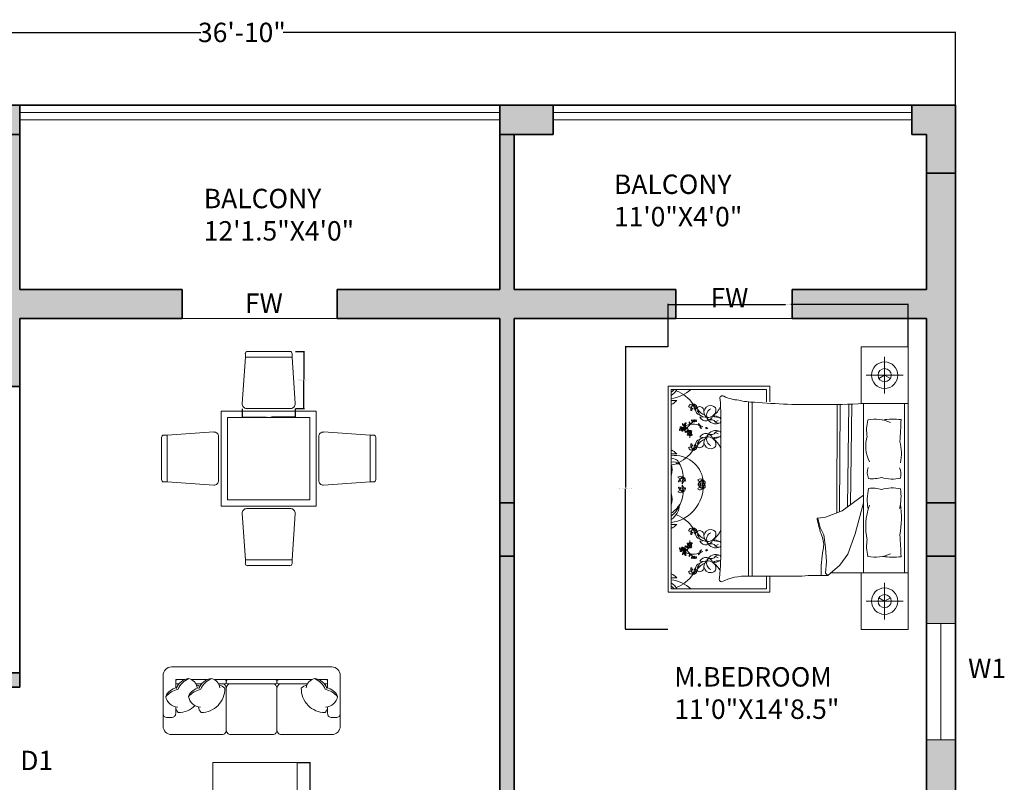
# Model space of a CAD drawing. Units: inches. Extents: x -9 to 505, y -680 to 48.
# Tile 17 of 17: x 179 to 484, y -198 to 38. Entities that reach past the tile are written whole.
import ezdxf

# ---------------------------------------------------------------- set-up
doc = ezdxf.new("R2010")
doc.units = ezdxf.units.IN
doc.header["$MEASUREMENT"] = 0
for name, color, linetype, lineweight in [('A-ANNO-DIMS', 2, 'Continuous', 18), ('A-ANNO-TEXT', 7, 'Continuous', 18), ('A-AREA-IDEN', 7, 'Continuous', 18), ('A-FLOR-HRAL', 4, 'Continuous', 18), ('A-FURN', 8, 'Continuous', 18), ('A-GLAZ', 4, 'Continuous', 18), ('A-WALL', 7, 'Continuous', 35), ('A-WALL-PATT', 251, 'Continuous', 13), ('S-CONC', 7, 'Continuous', 35), ('S-CONC-PATT', 18, 'Continuous', 13)]:
    doc.layers.add(name, color=color, linetype=linetype, lineweight=lineweight)
doc.styles.get("Standard").update_dxf_attribs({"font": 'arial.ttf'})
doc.dimstyles.get("Standard").update_dxf_attribs({"dimtxt": 0.18, "dimasz": 0.18, "dimexe": 0.18, "dimexo": 0.0625, "dimgap": 0.09, "dimtad": 0, "dimtih": 1, "dimtoh": 1, "dimdec": 0, "dimzin": 0, "dimdsep": 46, "dimlunit": 3, "dimtxsty": 'Standard', "dimcen": 0.09, "dimadec": 0, "dimazin": 0, "dimtfac": 1, "dimtdec": 0, "dimtofl": 0, "dimtmove": 0, "dimatfit": 3, "dimfxl": 1, "dimtolj": 1, "dimtzin": 0, "dimarcsym": 0})

# ---------------------------------------------------------------- blocks, each defined once
blk = doc.blocks.new('*D2')
at = {"layer": 'A-ANNO-DIMS', "color": 0, "lineweight": -2, "transparency": 16777216}
for p, q in [((27.26, 11.56), (27.26, 34.2)), ((27.44, 34.02), (235.29, 34.02)), ((468.58, 34.02), (260.74, 34.02)), ((468.76, 11.56), (468.76, 34.2))]:
    blk.add_line(p, q, dxfattribs=at)
at = {"layer": 'A-ANNO-DIMS', "color": 0, "transparency": 16777216}
for points in [[(27.44, 34.05), (27.44, 33.99), (27.26, 34.02)], [(468.58, 34.05), (468.58, 33.99), (468.76, 34.02)]]:
    blk.add_solid(points, dxfattribs=at)
at = {"layer": 'Defpoints', "color": 0, "transparency": 16777216}
for p in [(468.76, 34.02), (27.26, 11.5), (468.76, 11.5)]:
    blk.add_point(p, dxfattribs=at)
at = {"layer": 'A-ANNO-DIMS', "color": 0, "transparency": 16777216, "insert": (248.01, 34.02), "char_height": 6, "attachment_point": 5}
blk.add_mtext('\\A1;36\'-10"', dxfattribs=at)
blk = doc.blocks.new('BED-DOUBLE-WITH-NIGHTSTANDS')
for p, q in [((74.3, 0), (74.3, 87.37)), ((67.02, 72.93), (67.02, 84.34)), ((61.31, 78.63), (72.73, 78.63)), ((0, 75.23), (0, 11.53)), ((31.47, 75.23), (0, 75.23)), ((1.01, 74.22), (30.46, 74.22)), ((1.01, 12.54), (1.01, 74.22)), ((30.46, 74.22), (30.46, 70.37)), ((31.47, 70.38), (31.47, 75.23)), ((24.93, 70.38), (24.93, 16.47)), ((26.02, 70.29), (26.02, 16.47)), ((52.32, 69.59), (52.18, 36.06)), ((53.22, 69.58), (53.09, 36.41)), ((55.97, 69.63), (55.52, 37.9)), ((56.87, 69.66), (56.43, 38.56)), ((60.5, 17.47), (60.5, 69.9)), ((73.18, 69.9), (73.18, 17.47)), ((9.87, 65.61), (10.86, 65.8)), ((16.35, 61.42), (16.35, 25.95)), ((9.87, 59.5), (10.86, 59.31)), ((60.5, 41.48), (53.83, 36.69)), ((53.83, 36.69), (48.7, 34.74)), ((57.9, 29.61), (60.5, 39.14)), ((48.7, 34.74), (46.4, 34.39)), ((46.4, 34.39), (47.11, 31.56)), ((47.11, 31.56), (48.17, 29.26)), ((9.87, 27.26), (10.86, 27.45)), ((48.17, 29.26), (48.7, 25.36)), ((55.6, 23.24), (57.9, 29.61)), ((48.7, 25.36), (49.06, 20.94)), ((53.12, 19.88), (55.6, 23.24)), ((9.87, 21.15), (10.86, 20.96)), ((49.06, 20.94), (48.7, 17.4)), ((49.41, 16.69), (53.12, 19.88)), ((30.46, 16.47), (30.46, 12.54)), ((31.47, 11.53), (31.47, 16.47)), ((48.7, 17.4), (49.41, 16.69)), ((74.3, 17.47), (50.32, 17.47)), ((30.46, 12.54), (1.01, 12.54)), ((67.02, 14.45), (67.02, 3.03)), ((0, 11.53), (31.47, 11.53)), ((61.31, 8.74), (72.73, 8.74))]:
    blk.add_line(p, q)
for points in [[(74.3, 69.9), (59.74, 69.9), (59.74, 87.37), (74.3, 87.37)], [(67.02, 78.63), (65.26, 77.62)], [(67.02, 78.63), (68.79, 77.62)], [(59.74, 17.47), (59.74, 0), (74.3, 0)], [(67.02, 8.74), (65.26, 9.76)], [(67.02, 8.74), (68.79, 9.76)]]:
    blk.add_lwpolyline(points)
for points in [[(26.71, 70.27, -0.056112), (21.91, 70.9, -0.095341), (17.28, 72.13)], [(72.13, 64.88, 0.074897), (66.42, 64.77, -0.472817)], [(66.1, 47.01, 0.14099), (71.92, 46.83, 0.235245)], [(66.1, 43.28, -0.14099), (71.92, 43.45, -0.235245)], [(72.13, 22.49, -0.074897), (66.42, 22.6, 0.472817)], [(41.41, 16.51, -0.001242), (24.83, 16.47, 0.127202), (16.57, 14.72)]]:
    blk.add_lwpolyline(points, format="xyb")
for centre, radius in [((67.02, 78.63), 4.08), ((67.02, 78.63), 2.04), ((4.36, 62.02), 0.223), ((6.7, 60.56), 0.223), ((4.36, 24.75), 0.223), ((6.7, 26.2), 0.223), ((67.02, 8.74), 4.08), ((67.02, 8.74), 2.04)]:
    blk.add_circle(centre, radius)
for centre, radius, start, end in [((-2.05, 76.99), 5.56, 303.4617, 330.1116), ((-3.09, 78.99), 6.93, 306.3036, 316.4814), ((-0.53, 82.71), 11.41, 277.745, 311.8856), ((-1.65, 63.19), 11.41, 34.3865, 68.5908), ((-0.77, 73.87), 4.64, 292.5547, 318.9546), ((1.73, 86.58), 15.79, 267.4081, 273.6519), ((16.83, 71.47), 0.796, 56.1736, 203.4781), ((-68.63, 64.1), 85.02, 358.1965, 4.7598), ((44.11, 274.32), 204.79, 265.1265, 270.8855), ((7.49, 68.4), 1.27, 77.7115, 159.0387), ((6.81, 69.66), 0.953, 238.4633, 358.2869), ((9.93, 67.74), 2.89, 138.8402, 177.9352), ((7.19, 67.84), 0.142, 177.9352, 11.4834), ((7.26, 67.85), 0.0688, 11.4834, 127.9409), ((8.2, 68.81), 0.933, 117.6827, 223.7762), ((7.66, 68.26), 0.0744, 223.7729, 159.7333), ((7.99, 68.72), 0.946, 2.9516, 103.728), ((15.55, 71.37), 7.98, 192.5173, 207.1824), ((6.71, 68.17), 1.8, 345.4653, 54.2343), ((9.43, 70.65), 1.95, 211.3827, 255.2969), ((9.8, 67.61), 1.31, 350.264, 160.8688), ((10.19, 67.92), 1.64, 175.969, 254.3045), ((8.38, 67.88), 0.804, 333.9755, 53.2681), ((8.02, 66.16), 1.74, 6.1662, 51.5825), ((12.69, 70.21), 4.12, 211.2614, 251.7045), ((13.16, 67.13), 2.09, 84.9449, 172.8857), ((13.63, 67.49), 2.54, 182.3591, 234.0401), ((13.96, 66.31), 2.03, 111.5819, 201.4221), ((12.28, 68.18), 2.63, 265.2933, 346.921), ((13.37, 67.73), 1.48, 354.4856, 91.0538), ((10.2, 71.58), 6.61, 303.6671, 336.3547), ((49.82, 226.53), 156.99, 269.0718, 273.9), ((8.96, 64.13), 2.46, 178.3264, 187.1302), ((6.3, 63.79), 0.459, 11.3256, 64.4621), ((7.86, 64.45), 1.38, 190.2588, 210.656), ((1.29, 69.52), 8.3, 313.1541, 322.0459), ((7.39, 64.54), 0.171, 142.4737, 265.053), ((7.61, 64.57), 0.367, 127.7621, 169.0403), ((7.42, 64.88), 0.517, 265.053, 338.3618), ((8.1, 64.17), 0.676, 113.4276, 137.6104), ((8.03, 64.87), 0.223, 183.2768, 356.7232), ((8.19, 64.47), 0.364, 139.7889, 227.6792), ((8.07, 64.34), 0.192, 227.6792, 350.3487), ((7.33, 64.48), 0.728, 353.0852, 15.7171), ((7.81, 64.39), 0.46, 350.3487, 43.6538), ((8.66, 64.86), 0.535, 198.7263, 262.5032), ((8.24, 64.61), 0.213, 1.1081, 91.8675), ((8.64, 64.5), 0.172, 255.2356, 54.9248), ((8.37, 64.57), 0.371, 11.5637, 52.6358), ((12.35, 70.24), 4.69, 236.2883, 266.5076), ((11.75, 66.69), 2.17, 209.9085, 343.1337), ((12.67, 65.32), 0.542, 167.3041, 285.1471), ((14.13, 62.72), 3.37, 122.7011, 126.3445), ((14.77, 66.35), 2.78, 199.2822, 299.1751), ((13.28, 63.06), 1.79, 41.5653, 105.1471), ((15.71, 69.16), 3.62, 238.8218, 280.751), ((14.13, 62.72), 3.37, 55.785, 94.7304), ((14.26, 66.77), 2.51, 277.436, 299.9149), ((15.59, 65.12), 1.31, 221.5653, 293.8354), ((15.39, 64.67), 1.05, 17.4186, 52.325), ((15.39, 64.67), 1.05, 314.4517, 343.3657), ((73.15, 61.76), 11.71, 165.1039, 191.0369), ((64.13, 53.75), 11.26, 65.1316, 101.7583), ((903.62, 16.72), 832.89, 176.68521, 177.14978), ((3.72, 61.68), 0.171, 142.4737, 265.053), ((3.95, 61.71), 0.367, 61.2196, 169.0403), ((3.75, 62.02), 0.517, 265.053, 338.3618), ((4.19, 62.47), 0.439, 157.4086, 261.4386), ((3.94, 62.48), 0.22, 58.0499, 135.6268), ((4.44, 61.32), 0.676, 113.4276, 137.6104), ((4.17, 62.34), 0.147, 172.906, 277.132), ((3.69, 62.07), 0.702, 14.7558, 58.0499), ((4.52, 61.61), 0.364, 139.7889, 227.6792), ((4.41, 61.49), 0.192, 227.6792, 350.3487), ((4.67, 62.26), 0.303, 36.1046, 181.4281), ((3.66, 61.62), 0.728, 353.0852, 15.7171), ((4.68, 63.45), 0.248, 124.3538, 214.3923), ((4.14, 61.53), 0.46, 350.3487, 43.6538), ((5.05, 63.41), 0.579, 190.3057, 287.1958), ((4.49, 62.5), 0.306, 270.0645, 331.1507), ((4.75, 62.43), 0.35, 221.8413, 265.7877), ((4.99, 62.01), 0.535, 198.7263, 262.5032), ((5.21, 63.62), 0.673, 176.9701, 248.2913), ((10.01, 67.17), 6.5, 212.6784, 216.3746), ((4.57, 61.76), 0.213, 1.1081, 91.8675), ((4.75, 62.29), 0.218, 263.7526, 41.7054), ((4.7, 61.71), 0.371, 11.5637, 86.365), ((4.99, 63.46), 0.257, 216.3746, 291.7548), ((7.26, 59.85), 3.63, 124.0033, 132.4917), ((4.97, 61.64), 0.172, 255.2356, 54.9248), ((3.53, 59.39), 3.88, 63.7819, 68.2913), ((5.6, 62.38), 0.616, 128.3208, 208.8162), ((5.6, 63.28), 0.579, 122.8155, 187.3992), ((5.71, 62.42), 0.737, 207.7043, 254.3516), ((5.16, 63.04), 0.194, 289.3605, 111.7548), ((5.3, 63.04), 0.194, 221.8703, 44.2646), ((6.18, 62.48), 1.01, 157.2305, 229.0635), ((5.86, 63.21), 0.673, 109.4799, 177.6828), ((5.84, 62.81), 0.597, 174.4544, 220.6188), ((5.23, 62), 1.01, 270.278, 342.111), ((5.91, 60.73), 0.717, 98.7227, 159.3375), ((5.55, 61.65), 0.737, 244.9899, 291.6373), ((2.45, 59.48), 4.35, 30.544, 49.818), ((5.5, 63.63), 0.248, 56.8636, 146.9021), ((5.62, 63.36), 0.257, 148.8844, 224.2646), ((4.84, 61.96), 0.717, 340.0041, 40.6188), ((10.97, 60.13), 6.5, 145.1882, 148.8844), ((7.26, 59.85), 3.63, 94.756, 119.2041), ((14.99, 54.63), 11.94, 132.2412, 142.1744), ((5.71, 62.03), 0.597, 278.7227, 324.8872), ((5.61, 61.55), 0.616, 290.5253, 358.5375), ((6.53, 61.01), 0.439, 157.4086, 261.4386), ((6.29, 61.03), 0.22, 58.0499, 135.6268), ((6.81, 61.72), 0.616, 182.8499, 266.1226), ((6.57, 62.16), 0.597, 231.7607, 277.9252), ((7.04, 62.26), 1.01, 214.5369, 286.3699), ((6.03, 60.62), 0.702, 14.7558, 58.0499), ((2.45, 59.48), 4.35, 23.0501, 23.8477), ((6.93, 63.89), 0.419, 188.3432, 274.2869), ((6.75, 60.86), 0.717, 37.3105, 97.9252), ((7.3, 64.12), 0.732, 210.656, 242.6341), ((7.01, 60.81), 0.303, 36.1046, 181.4281), ((7.85, 64.75), 1.4, 218.2101, 226.3071), ((6.83, 61.84), 0.737, 265.0106, 311.658), ((6.82, 63.57), 0.178, 325.7657, 67.4417), ((7.45, 56.25), 7.24, 73.5842, 93.8277), ((7.1, 60.84), 0.218, 263.7526, 41.7054), ((11.9, 63.61), 2.46, 178.3264, 187.1302), ((9.24, 63.27), 0.459, 11.3256, 64.4621), ((10.8, 63.93), 1.38, 190.2588, 210.656), ((9.87, 63.37), 0.419, 188.3432, 274.2869), ((10.24, 63.6), 0.732, 210.656, 242.6341), ((10.79, 64.23), 1.4, 218.2101, 226.3071), ((9.76, 63.05), 0.178, 325.7657, 67.4417), ((10.26, 62.72), 0.419, 147.5332, 233.4768), ((10.63, 62.94), 0.732, 179.1859, 211.164), ((9.92, 62.77), 0.178, 354.3784, 96.0543), ((7.45, 56.25), 7.24, 63.0032, 69.8941), ((11.19, 63.27), 1.38, 211.164, 231.5612), ((11.43, 64.4), 2.46, 234.6898, 243.4936), ((11.45, 63.13), 1.4, 195.5129, 203.6099), ((9.87, 62.21), 0.459, 357.3579, 50.4944), ((11.84, 62.3), 0.168, 12.7051, 190.4384), ((11.95, 62.32), 0.274, 190.4384, 10.4136), ((14.77, 58.76), 2.78, 60.8249, 160.7178), ((15.59, 59.99), 1.31, 66.1646, 138.4347), ((15.39, 60.44), 1.05, 23.2856, 45.5483), ((6.07, 60.22), 0.171, 142.4737, 265.053), ((6.29, 60.26), 0.367, 61.2196, 169.0403), ((6.1, 60.57), 0.517, 265.053, 338.3618), ((6.78, 59.86), 0.676, 113.4276, 137.6104), ((6.52, 60.89), 0.147, 172.906, 277.132), ((6.87, 60.16), 0.364, 139.7889, 227.6792), ((6.75, 60.03), 0.192, 227.6792, 350.3487), ((6.01, 60.16), 0.728, 353.0852, 15.7171), ((2.45, 59.48), 4.35, 357.1071, 4.7585), ((6.49, 60.07), 0.46, 350.3487, 43.6538), ((7.34, 60.55), 0.535, 198.7263, 262.5032), ((6.84, 61.04), 0.306, 270.0645, 331.1507), ((7.1, 60.97), 0.35, 221.8413, 265.7877), ((6.91, 60.3), 0.213, 1.1081, 91.8675), ((7.05, 60.25), 0.371, 11.5637, 86.365), ((7.31, 60.19), 0.172, 255.2356, 54.9248), ((10.19, 57.19), 1.64, 105.6955, 184.031), ((8.02, 58.95), 1.74, 308.4175, 353.8338), ((12.69, 54.9), 4.12, 108.2955, 148.7386), ((12.35, 54.86), 4.69, 93.4924, 123.7117), ((11.75, 58.42), 2.17, 16.8663, 150.0915), ((13.63, 57.62), 2.54, 125.9599, 177.6409), ((13.96, 58.8), 2.03, 158.5779, 248.4181), ((12.28, 56.93), 2.63, 13.079, 94.7067), ((12.67, 59.79), 0.542, 74.8529, 192.6959), ((14.13, 62.39), 3.37, 233.6555, 237.2989), ((13.28, 62.05), 1.79, 254.8529, 318.4347), ((15.71, 55.95), 3.62, 79.7133, 121.1782), ((14.13, 62.39), 3.37, 265.2696, 304.215), ((10.2, 53.53), 6.61, 21.4941, 56.3329), ((14.26, 58.33), 2.51, 60.0851, 82.564), ((15.39, 60.44), 1.05, 307.675, 336.7144), ((72.29, 56.71), 11.12, 163.8254, 206.1239), ((56.84, 54.51), 15.36, 348.8159, 13.6573), ((-0.77, 51.23), 4.64, 41.0454, 67.4453), ((-1.65, 61.92), 11.41, 291.4092, 325.6135), ((6.81, 55.44), 0.953, 1.7131, 121.5367), ((7.49, 56.71), 1.27, 200.9613, 282.2885), ((7.19, 57.27), 0.142, 348.5166, 182.0648), ((9.93, 57.37), 2.89, 182.0648, 221.1598), ((7.26, 57.26), 0.0688, 232.0591, 348.5166), ((8.2, 56.3), 0.933, 136.2238, 242.3173), ((7.61, 56.86), 0.123, 200.2817, 136.2238), ((6.71, 56.94), 1.8, 305.7657, 14.5347), ((15.55, 53.74), 7.98, 152.8176, 167.4827), ((7.99, 56.39), 0.946, 256.272, 357.0484), ((9.43, 54.46), 1.95, 104.7031, 148.6173), ((9.8, 57.5), 1.31, 199.1312, 9.736), ((8.38, 57.23), 0.804, 306.7319, 26.0245), ((13.16, 57.98), 2.09, 187.1143, 275.0551), ((13.37, 57.38), 1.48, 268.9462, 5.5144), ((1.73, 38.53), 15.79, 86.3481, 92.5919), ((2.11, 44.94), 8.83, 8.1803, 97.1364), ((1.49, 50.77), 2.05, 10.9261, 103.6102), ((1.78, 49.23), 2.59, 48.0951, 107.1391), ((-4.99, 49.37), 6.27, 343.5431, 17.0202), ((2.92, 46.08), 5.11, 83.3805, 111.883), ((-6.64, 46.18), 11.41, 4.4623, 27.4146), ((66.26, 48.62), 4.63, 161.4593, 204.9817), ((67.77, 48.03), 4.32, 343.8974, 26.6563), ((-8.22, 46.89), 9.28, 4.3787, 5.6357), ((-14.58, 42), 16.58, 19.7217, 19.9028), ((3.89, 46.13), 1.27, 47.7873, 129.1145), ((3.93, 47.57), 0.953, 208.5391, 328.3627), ((3.35, 45.79), 0.142, 148.011, 341.5592), ((5.67, 44.34), 2.89, 108.9159, 148.011), ((3.42, 45.77), 0.0688, 341.5592, 98.0167), ((4.7, 46.14), 0.933, 87.7585, 193.852), ((3.96, 45.93), 0.0744, 193.9791, 129.8091), ((12.35, 44.68), 7.98, 162.593, 177.2582), ((3.09, 46.33), 1.8, 315.5411, 24.3101), ((6.69, 47.12), 1.95, 181.4585, 225.3727), ((4.47, 46.16), 0.946, 333.0274, 73.8037), ((10, 45.26), 1.27, 47.7873, 129.1145), ((10.04, 46.7), 0.953, 208.5391, 328.3627), ((11.79, 43.47), 2.89, 108.9159, 148.011), ((10.81, 45.26), 0.933, 87.7585, 193.852), ((9.21, 45.45), 1.8, 315.5411, 24.3101), ((18.47, 43.81), 7.98, 162.593, 177.2582), ((10.59, 45.29), 0.946, 333.0274, 73.8037), ((12.8, 46.25), 1.95, 181.4585, 225.3727), ((63.18, 57.31), 10.71, 264.0129, 285.8293), ((-0.53, 44.37), 11.41, 277.745, 355.5377), ((3.93, 42.1), 0.953, 31.6373, 151.4609), ((3.35, 43.88), 0.142, 18.4408, 211.989), ((5.67, 45.33), 2.89, 211.989, 251.0841), ((3.42, 43.9), 0.0688, 261.9833, 18.4408), ((4.7, 43.54), 0.933, 166.148, 272.2415), ((3.92, 43.73), 0.123, 230.0755, 166.148), ((12.35, 44.99), 7.98, 182.7418, 197.407), ((3.09, 43.35), 1.8, 335.6899, 44.4589), ((6.69, 42.55), 1.95, 134.6273, 178.5415), ((4.47, 43.51), 0.946, 286.1963, 26.9726), ((10.04, 42.98), 0.953, 31.6373, 151.4609), ((10, 44.41), 1.27, 230.8855, 312.2127), ((9.46, 44.92), 0.142, 148.011, 341.5592), ((9.46, 44.75), 0.142, 18.4408, 211.989), ((11.79, 46.21), 2.89, 211.989, 251.0841), ((9.53, 44.9), 0.0688, 341.5592, 98.0167), ((9.53, 44.78), 0.0688, 261.9833, 18.4408), ((10.81, 44.41), 0.933, 166.148, 272.2415), ((10.03, 44.6), 0.123, 230.0755, 166.148), ((10.07, 45.06), 0.0744, 193.9791, 129.8091), ((9.21, 44.22), 1.8, 335.6899, 44.4589), ((18.47, 45.87), 7.98, 182.7418, 197.407), ((10.59, 44.39), 0.946, 286.1963, 26.9726), ((12.8, 43.43), 1.95, 134.6273, 178.5415), ((77.04, 40), 15.41, 166.3762, 190.1383), ((63.18, 32.98), 10.71, 74.1707, 95.9871), ((56.52, 41.16), 15.57, 346.04, 8.4751), ((-4.99, 40.3), 6.27, 342.9798, 16.4569), ((-8.22, 42.79), 9.28, 354.3643, 355.6213), ((-14.58, 47.67), 16.58, 340.0972, 340.2783), ((3.89, 43.54), 1.27, 230.8855, 312.2127), ((-6.64, 43.49), 11.41, 332.5854, 355.5377), ((-2.05, 38.64), 5.56, 303.4617, 358.728), ((-5.04, 44.28), 10.31, 305.947, 325.9877), ((-3.09, 40.64), 6.93, 306.3036, 342.1496), ((81.47, 31.77), 20.31, 160.7385, 191.9603), ((40.51, 34.46), 31.69, 350.503, 7.7804), ((-1.65, 24.85), 11.41, 34.3865, 68.5908), ((46.33, 34.19), 0.211, 70.2464, 181.1377), ((79.42, 40.46), 33.88, 190.6617, 199.8806), ((1.73, 48.24), 15.79, 267.4081, 273.6519), ((-0.77, 35.53), 4.64, 292.5547, 318.9546), ((7.49, 30.05), 1.27, 77.7115, 159.0387), ((6.81, 31.32), 0.953, 238.4633, 358.2869), ((9.93, 29.39), 2.89, 138.8402, 177.9352), ((8.2, 30.46), 0.933, 117.6827, 223.7762), ((7.99, 30.37), 0.946, 2.9516, 103.728), ((9.43, 32.3), 1.95, 211.3827, 255.2969), ((6.71, 29.83), 1.8, 345.4653, 54.2343), ((15.55, 33.02), 7.98, 192.5173, 207.1824), ((9.8, 29.26), 1.31, 350.264, 160.8688), ((13.16, 28.78), 2.09, 84.9449, 172.8857), ((13.37, 29.38), 1.48, 354.4856, 91.0538), ((10.2, 33.24), 6.61, 303.6671, 338.5059), ((2.45, 27.28), 4.35, 355.2415, 2.8929), ((7.19, 29.49), 0.142, 177.9352, 11.4834), ((7.26, 29.5), 0.0688, 11.4834, 127.9409), ((7.66, 29.92), 0.0744, 223.7729, 159.7333), ((10.19, 29.57), 1.64, 175.969, 254.3045), ((8.38, 29.53), 0.804, 333.9755, 53.2681), ((8.02, 27.81), 1.74, 6.1662, 51.5825), ((12.69, 31.86), 4.12, 211.2614, 251.7045), ((12.35, 31.9), 4.69, 236.2883, 266.5076), ((11.75, 28.34), 2.17, 209.9085, 343.1337), ((13.63, 29.14), 2.54, 182.3591, 234.0401), ((13.96, 27.96), 2.03, 111.5819, 201.4221), ((12.28, 29.84), 2.63, 265.2933, 346.921), ((15.71, 30.81), 3.62, 238.8218, 280.2867), ((14.13, 24.37), 3.37, 55.785, 94.7304), ((41.05, 26.07), 7.11, 348.6608, 23.7384), ((73.15, 25.61), 11.71, 168.9631, 194.8961), ((903.62, 70.65), 832.89, 182.85022, 183.31479), ((3.72, 25.08), 0.171, 94.947, 217.5263), ((3.95, 25.05), 0.367, 190.9597, 298.7804), ((3.75, 24.74), 0.517, 21.6382, 94.947), ((4.19, 24.29), 0.439, 98.5614, 202.5914), ((4.44, 25.45), 0.676, 222.3896, 246.5724), ((4.17, 24.42), 0.147, 82.868, 187.094), ((3.69, 24.69), 0.702, 301.9501, 345.2442), ((4.52, 25.15), 0.364, 132.3208, 220.2111), ((4.41, 25.28), 0.192, 9.6513, 132.3208), ((3.66, 25.14), 0.728, 344.2829, 6.9148), ((4.67, 24.5), 0.303, 178.5719, 323.8954), ((4.14, 25.23), 0.46, 316.3462, 9.6513), ((4.99, 24.76), 0.535, 97.4968, 161.2737), ((4.75, 24.34), 0.35, 94.2123, 138.1587), ((4.49, 24.26), 0.306, 28.8493, 89.9355), ((4.57, 25.01), 0.213, 268.1325, 358.8919), ((4.7, 25.05), 0.371, 273.635, 348.4363), ((4.75, 24.47), 0.218, 318.2946, 96.2474), ((4.97, 25.12), 0.172, 305.0752, 104.7644), ((5.6, 24.39), 0.616, 151.1838, 231.6792), ((5.71, 24.34), 0.737, 105.6484, 152.2957), ((6.18, 24.28), 1.01, 130.9365, 202.7695), ((5.55, 25.11), 0.737, 68.3627, 115.0101), ((5.23, 24.76), 1.01, 17.889, 89.722), ((5.91, 26.03), 0.717, 200.6625, 261.2773), ((2.45, 27.28), 4.35, 310.182, 329.456), ((4.84, 24.8), 0.717, 319.3812, 19.9959), ((14.99, 32.13), 11.94, 217.8256, 227.7588), ((5.71, 24.73), 0.597, 35.1128, 81.2773), ((5.61, 25.22), 0.616, 1.4625, 69.4747), ((6.07, 26.54), 0.171, 94.947, 217.5263), ((6.29, 26.51), 0.367, 190.9597, 298.7804), ((6.1, 26.19), 0.517, 21.6382, 94.947), ((6.53, 25.75), 0.439, 98.5614, 202.5914), ((6.29, 25.74), 0.22, 224.3732, 301.9501), ((6.81, 25.04), 0.616, 93.8774, 177.1501), ((7.04, 24.5), 1.01, 73.6301, 145.4631), ((6.57, 24.61), 0.597, 82.0748, 128.2393), ((6.78, 26.9), 0.676, 222.3896, 246.5724), ((6.52, 25.87), 0.147, 82.868, 187.094), ((6.03, 26.14), 0.702, 301.9501, 345.2442), ((2.45, 27.28), 4.35, 336.1523, 336.9499), ((6.87, 26.61), 0.364, 132.3208, 220.2111), ((6.75, 26.73), 0.192, 9.6513, 132.3208), ((6.75, 25.91), 0.717, 262.0748, 322.6895), ((6.01, 26.6), 0.728, 344.2829, 6.9148), ((7.01, 25.96), 0.303, 178.5719, 323.8954), ((6.83, 24.92), 0.737, 48.342, 94.9894), ((6.49, 26.69), 0.46, 316.3462, 9.6513), ((7.34, 26.21), 0.535, 97.4968, 161.2737), ((7.1, 25.79), 0.35, 94.2123, 138.1587), ((6.84, 25.72), 0.306, 28.8493, 89.9355), ((6.91, 26.46), 0.213, 268.1325, 358.8919), ((7.05, 26.51), 0.371, 273.635, 348.4363), ((7.1, 25.92), 0.218, 318.2946, 96.2474), ((7.31, 26.58), 0.172, 305.0752, 104.7644), ((10.26, 24.04), 0.419, 126.5232, 212.4668), ((11.19, 23.49), 1.38, 128.4388, 148.836), ((11.43, 22.37), 2.46, 116.5064, 125.3102), ((9.87, 24.55), 0.459, 309.5056, 2.6421), ((11.95, 24.44), 0.274, 349.5864, 169.5616), ((11.84, 24.46), 0.168, 169.5616, 347.2949), ((12.67, 26.97), 0.542, 167.3041, 285.1471), ((14.13, 24.37), 3.37, 122.7011, 126.3445), ((14.77, 28.01), 2.78, 199.2822, 299.1751), ((13.28, 24.72), 1.79, 41.5653, 105.1471), ((14.26, 28.43), 2.51, 277.436, 299.9149), ((15.59, 26.77), 1.31, 221.5653, 293.8354), ((-74.6, 24.91), 90.96, 354.3113, 0.6567), ((15.39, 26.33), 1.05, 23.2856, 52.325), ((15.39, 26.33), 1.05, 314.4517, 336.771), ((80.35, 18.19), 32.98, 168.6608, 182.5481), ((3.94, 24.28), 0.22, 224.3732, 301.9501), ((4.68, 23.31), 0.248, 145.6077, 235.6462), ((5.05, 23.35), 0.579, 72.8042, 169.6943), ((5.21, 23.14), 0.673, 111.7087, 183.0299), ((10.01, 19.6), 6.5, 143.6254, 147.3216), ((4.99, 23.3), 0.257, 68.2452, 143.6254), ((7.26, 26.91), 3.63, 227.5083, 235.9967), ((3.53, 27.37), 3.88, 291.7087, 296.2181), ((5.6, 23.48), 0.579, 172.6008, 237.1845), ((5.16, 23.72), 0.194, 248.2452, 70.6395), ((5.3, 23.72), 0.194, 315.7354, 138.1297), ((5.86, 23.55), 0.673, 182.3172, 250.5201), ((5.84, 23.95), 0.597, 139.3812, 185.5456), ((5.5, 23.13), 0.248, 213.0979, 303.1364), ((5.62, 23.4), 0.257, 135.7354, 211.1156), ((10.97, 26.63), 6.5, 211.1156, 214.8118), ((7.26, 26.91), 3.63, 240.7959, 265.244), ((7.86, 22.31), 1.38, 149.344, 169.7412), ((8.96, 22.63), 2.46, 172.8698, 181.6736), ((6.3, 22.97), 0.459, 295.5379, 348.6744), ((6.93, 22.88), 0.419, 85.7131, 171.6568), ((7.3, 22.64), 0.732, 117.3659, 149.344), ((7.85, 22.01), 1.4, 133.6929, 141.7899), ((6.82, 23.19), 0.178, 292.5583, 34.2343), ((7.45, 30.51), 7.24, 266.1723, 286.4158), ((1.29, 17.24), 8.3, 37.9541, 46.8459), ((7.39, 22.23), 0.171, 94.947, 217.5263), ((7.61, 22.19), 0.367, 190.9597, 232.2379), ((7.42, 21.88), 0.517, 21.6382, 94.947), ((8.1, 22.59), 0.676, 222.3896, 246.5724), ((8.03, 21.89), 0.223, 3.2768, 176.7232), ((8.19, 22.29), 0.364, 132.3208, 220.2111), ((8.07, 22.42), 0.192, 9.6513, 132.3208), ((7.33, 22.29), 0.728, 344.2829, 6.9148), ((7.81, 22.37), 0.46, 316.3462, 9.6513), ((8.66, 21.9), 0.535, 97.4968, 161.2737), ((8.24, 22.15), 0.213, 268.1325, 358.8919), ((8.64, 22.26), 0.172, 305.0752, 104.7644), ((8.37, 22.2), 0.371, 307.3642, 348.4363), ((10.8, 22.83), 1.38, 149.344, 169.7412), ((11.9, 23.15), 2.46, 172.8698, 181.6736), ((9.24, 23.49), 0.459, 295.5379, 348.6744), ((9.87, 23.4), 0.419, 85.7131, 171.6568), ((10.24, 23.16), 0.732, 117.3659, 149.344), ((10.79, 22.54), 1.4, 133.6929, 141.7899), ((9.76, 23.71), 0.178, 292.5583, 34.2343), ((11.75, 20.07), 2.17, 16.8663, 150.0915), ((10.63, 23.83), 0.732, 148.836, 180.8141), ((9.92, 23.99), 0.178, 263.9457, 5.6216), ((7.45, 30.51), 7.24, 290.1059, 296.9968), ((11.45, 23.63), 1.4, 156.3901, 164.4871), ((13.63, 19.27), 2.54, 125.9599, 177.6409), ((12.67, 21.45), 0.542, 74.8529, 192.6959), ((14.77, 20.41), 2.78, 60.8249, 160.7178), ((14.13, 24.04), 3.37, 233.6555, 237.2989), ((13.28, 23.7), 1.79, 254.8529, 318.4347), ((14.26, 19.99), 2.51, 60.0851, 82.564), ((15.59, 21.64), 1.31, 66.1646, 138.4347), ((15.39, 22.09), 1.05, 307.675, 329.9707), ((15.39, 22.09), 1.05, 26.442, 45.5483), ((64.13, 33.62), 11.26, 258.2417, 294.8684), ((7.19, 18.93), 0.142, 348.5166, 182.0648), ((9.93, 19.03), 2.89, 182.0648, 221.1598), ((7.26, 18.91), 0.0688, 232.0591, 348.5166), ((8.2, 17.95), 0.933, 136.2238, 242.3173), ((7.61, 18.51), 0.123, 200.2817, 136.2238), ((15.55, 15.4), 7.98, 152.8176, 167.4827), ((6.71, 18.59), 1.8, 305.7657, 14.5347), ((10.19, 18.84), 1.64, 105.6955, 184.031), ((9.8, 19.16), 1.31, 199.1312, 9.736), ((8.38, 18.89), 0.804, 306.7319, 26.0245), ((8.02, 20.61), 1.74, 308.4175, 353.8338), ((12.69, 16.56), 4.12, 108.2955, 148.7386), ((12.35, 16.52), 4.69, 93.4924, 123.7117), ((13.16, 19.64), 2.09, 187.1143, 275.0551), ((13.96, 20.46), 2.03, 158.5779, 248.4181), ((12.28, 18.58), 2.63, 13.079, 94.7067), ((13.37, 19.03), 1.48, 268.9462, 5.5144), ((15.71, 17.61), 3.62, 80.8446, 121.1782), ((14.13, 24.04), 3.37, 265.2696, 304.215), ((10.2, 15.18), 6.61, 26.7003, 56.3329), ((-0.77, 12.89), 4.64, 41.0454, 67.4453), ((1.73, 0.18), 15.79, 86.3481, 92.5919), ((-0.53, 4.05), 11.41, 48.1144, 82.255), ((-1.65, 23.57), 11.41, 291.4092, 325.6135), ((6.81, 17.1), 0.953, 1.7131, 121.5367), ((7.49, 18.36), 1.27, 200.9613, 282.2885), ((9.43, 16.11), 1.95, 104.7031, 148.6173), ((7.99, 18.05), 0.946, 256.272, 357.0484), ((16.63, 15.52), 0.806, 152.6588, 266.02), ((47.24, -63.42), 80.14, 88.447, 94.1706), ((-2.05, 9.77), 5.56, 29.8884, 56.5383), ((-3.09, 7.77), 6.93, 43.5186, 53.6964)]:
    blk.add_arc(centre, radius, start, end)
blk = doc.blocks.new('WIN-36')
for p, q in [((0, 36), (0, 0)), ((9, 36), (0, 36)), ((4.5, 36), (4.5, 2.23)), ((9, 0), (9, 36)), ((0, 0), (9, 0)), ((4.5, 2.23), (4.5, 0))]:
    blk.add_line(p, q)
blk = doc.blocks.new('CHAIR-DINING-ROUNDED')
for p, q in [((0, 1.49), (0.98, 15.88)), ((0.98, 16.94), (0.98, 15.88)), ((15.44, 15.88), (0.98, 15.88)), ((14.74, 17.64), (1.68, 17.64)), ((15.44, 15.88), (15.44, 16.94)), ((15.44, 15.88), (16.42, 1.49)), ((1.41, 0), (15.01, 0))]:
    blk.add_line(p, q)
for centre, radius, start, end in [((1.68, 16.94), 0.706, 90, 180), ((14.74, 16.94), 0.706, 0, 90), ((1.41, 1.41), 1.41, 176.8779, 270), ((15.01, 1.41), 1.41, 270, 3.1221)]:
    blk.add_arc(centre, radius, start, end)
blk = doc.blocks.new('TABLE-COFFEE-SQUARE')
at = {"ltscale": 0.03}
blk.add_lwpolyline([(0, 0), (26.11, 0), (26.11, 26.11), (0, 26.11)], close=True, dxfattribs=at)
blk = doc.blocks.new('*D20')
at = {"layer": 'A-ANNO-DIMS', "color": 0, "lineweight": -2, "transparency": 16777216}
for p, q in [((379.77, -63.25), (366.55, -63.25)), ((366.73, -63.43), (366.73, -106.76)), ((366.73, -150.44), (366.73, -107.12)), ((379.77, -150.62), (366.55, -150.62))]:
    blk.add_line(p, q, dxfattribs=at)
at = {"layer": 'A-ANNO-DIMS', "color": 0, "transparency": 16777216}
for points in [[(366.7, -63.43), (366.76, -63.43), (366.73, -63.25)], [(366.7, -150.44), (366.76, -150.44), (366.73, -150.62)]]:
    blk.add_solid(points, dxfattribs=at)
at = {"layer": 'Defpoints', "color": 0, "transparency": 16777216}
for p in [(366.73, -63.25), (379.83, -63.25), (379.83, -150.62)]:
    blk.add_point(p, dxfattribs=at)
at = {"layer": 'A-ANNO-DIMS', "color": 0, "transparency": 16777216, "insert": (366.73, -106.94), "char_height": 0.18, "attachment_point": 5}
blk.add_mtext('\\A1;BED & NIGHTSTANDS 7\'-3 1/2" TYP.', dxfattribs=at)
blk = doc.blocks.new('*D21')
at = {"layer": 'A-ANNO-DIMS', "color": 0, "lineweight": -2, "transparency": 16777216}
for p, q in [((379.83, -63.19), (379.83, -49.97)), ((380.01, -50.15), (416.13, -50.15)), ((453.95, -50.15), (417.83, -50.15)), ((454.13, -63.19), (454.13, -49.97))]:
    blk.add_line(p, q, dxfattribs=at)
at = {"layer": 'A-ANNO-DIMS', "color": 0, "transparency": 16777216}
for points in [[(380.01, -50.12), (380.01, -50.18), (379.83, -50.15)], [(453.95, -50.12), (453.95, -50.18), (454.13, -50.15)]]:
    blk.add_solid(points, dxfattribs=at)
at = {"layer": 'Defpoints', "color": 0, "transparency": 16777216}
for p in [(454.13, -50.15), (379.83, -63.25), (454.13, -63.25)]:
    blk.add_point(p, dxfattribs=at)
at = {"layer": 'A-ANNO-DIMS', "color": 0, "transparency": 16777216, "insert": (416.98, -50.15), "char_height": 0.18, "attachment_point": 5}
blk.add_mtext('\\A1;6\'-2 1/2" TYP.', dxfattribs=at)
blk = doc.blocks.new('*D39')
at = {"layer": 'A-ANNO-DIMS', "color": 0, "lineweight": -2, "transparency": 16777216}
for p, q in [((265.2, -191.76), (269.23, -191.76)), ((269.05, -191.94), (269.05, -204.64)), ((269.05, -217.69), (269.05, -205)), ((265.2, -217.87), (269.23, -217.87))]:
    blk.add_line(p, q, dxfattribs=at)
at = {"layer": 'A-ANNO-DIMS', "color": 0, "transparency": 16777216}
for points in [[(269.02, -191.94), (269.08, -191.94), (269.05, -191.76)], [(269.02, -217.69), (269.08, -217.69), (269.05, -217.87)]]:
    blk.add_solid(points, dxfattribs=at)
at = {"layer": 'Defpoints', "color": 0, "transparency": 16777216}
for p in [(265.13, -191.76), (269.05, -191.76), (265.13, -217.87)]:
    blk.add_point(p, dxfattribs=at)
at = {"layer": 'A-ANNO-DIMS', "color": 0, "transparency": 16777216, "insert": (269.05, -204.82), "char_height": 0.18, "attachment_point": 5}
blk.add_mtext('\\A1;2\'-2" TYP.', dxfattribs=at)
blk = doc.blocks.new('*D42')
at = {"layer": 'A-ANNO-DIMS', "color": 0, "lineweight": -2, "transparency": 16777216}
for p, q in [((264.59, -64.64), (267.36, -64.64)), ((267.18, -64.82), (267.18, -73.28)), ((267.18, -82.11), (267.18, -73.65)), ((264.59, -82.29), (267.36, -82.29))]:
    blk.add_line(p, q, dxfattribs=at)
at = {"layer": 'A-ANNO-DIMS', "color": 0, "transparency": 16777216}
for points in [[(267.15, -64.82), (267.21, -64.82), (267.18, -64.64)], [(267.15, -82.11), (267.21, -82.11), (267.18, -82.29)]]:
    blk.add_solid(points, dxfattribs=at)
at = {"layer": 'Defpoints', "color": 0, "transparency": 16777216}
for p in [(264.53, -64.64), (267.18, -64.64), (264.53, -82.29)]:
    blk.add_point(p, dxfattribs=at)
at = {"layer": 'A-ANNO-DIMS', "color": 0, "transparency": 16777216, "insert": (267.18, -73.46), "char_height": 0.18, "attachment_point": 5}
blk.add_mtext('\\A1;DINING CHAIR 1\'-5 1/2" TYP.', dxfattribs=at)
blk = doc.blocks.new('*D43')
at = {"layer": 'A-ANNO-DIMS', "color": 0, "lineweight": -2, "transparency": 16777216}
for p, q in [((248.07, -82.35), (248.07, -85.11)), ((248.25, -84.93), (255.46, -84.93)), ((264.35, -84.93), (257.14, -84.93)), ((264.53, -82.35), (264.53, -85.11))]:
    blk.add_line(p, q, dxfattribs=at)
at = {"layer": 'A-ANNO-DIMS', "color": 0, "transparency": 16777216}
for points in [[(248.25, -84.9), (248.25, -84.96), (248.07, -84.93)], [(264.35, -84.9), (264.35, -84.96), (264.53, -84.93)]]:
    blk.add_solid(points, dxfattribs=at)
at = {"layer": 'Defpoints', "color": 0, "transparency": 16777216}
for p in [(248.07, -82.29), (264.53, -82.29), (264.53, -84.93)]:
    blk.add_point(p, dxfattribs=at)
at = {"layer": 'A-ANNO-DIMS', "color": 0, "transparency": 16777216, "insert": (256.3, -84.93), "char_height": 0.18, "attachment_point": 5}
blk.add_mtext('\\A1;1\'-4 1/2" TYP.', dxfattribs=at)

msp = doc.modelspace()

# ---------------------------------------------------------------- hatches: boundary and pattern name
at = {"layer": 'A-WALL-PATT'}
h = msp.add_hatch(color=256, dxfattribs=at)
h.dxf.hatch_style = 1
h.paths.add_polyline_path([(101.64, 11.5), (48.26, 11.5), (48.26, 2.5), (72.26, 2.5), (72.26, -21.25), (81.26, -21.25), (81.26, 2.5), (101.64, 2.5)])
h.paths.add_polyline_path([(36.26, 2.5), (27.26, 2.5), (27.26, -6.92), (36.26, -6.92)])
h.paths.add_polyline_path([(81.26, -57.25), (72.26, -57.25), (72.26, -75.5), (81.26, -75.5)])
h.paths.add_polyline_path([(162.76, 11.5), (137.64, 11.5), (137.64, 2.5), (162.76, 2.5)])
h.paths.add_polyline_path([(179.26, 2.5), (174.76, 2.5), (174.76, -75.5), (179.26, -75.5), (179.26, -54.5), (229.51, -54.5), (229.51, -45.5), (179.26, -45.5)])
h.paths.add_polyline_path([(382.26, -45.5), (332.26, -45.5), (332.26, 2.5), (327.76, 2.5), (327.76, -45.5), (277.51, -45.5), (277.51, -54.5), (327.76, -54.5), (327.76, -111.5), (332.26, -111.5), (332.26, -54.5), (382.26, -54.5)])
h.paths.add_polyline_path([(332.26, -128), (327.76, -128), (327.76, -207), (332.26, -207)])
h.paths.add_polyline_path([(124.76, -111.5), (36.26, -111.5), (36.26, -116), (120.26, -116), (120.26, -168.5), (179.26, -168.5), (179.26, -164), (124.76, -164)])
h.paths.add_polyline_path([(96.26, -164), (36.26, -164), (36.26, -152), (27.26, -152), (27.26, -208.88), (36.26, -208.88), (36.26, -168.5), (96.26, -168.5)])
h.paths.add_polyline_path([(36.26, -244.88), (27.26, -244.88), (27.26, -287), (36.26, -287)])
h.paths.add_polyline_path([(179.26, -204.5), (174.76, -204.5), (174.76, -287), (179.26, -287)])
h.paths.add_polyline_path([(257.26, -296), (248.26, -296), (248.26, -446), (269.26, -446), (269.26, -437), (257.26, -437)])
h.paths.add_polyline_path([(90.26, -296), (81.26, -296), (81.26, -348.67), (90.26, -348.67)])
h.paths.add_polyline_path([(90.26, -384.67), (81.26, -384.67), (81.26, -416), (90.26, -416)])
h.paths.add_polyline_path([(170.26, -452), (36.26, -452), (36.26, -456.5), (165.76, -456.5), (165.76, -504.5), (165.13, -504.5), (165.13, -509), (170.26, -509)])
h.paths.add_polyline_path([(141.76, -504.5), (36.26, -504.5), (36.26, -492.5), (27.26, -492.5), (27.26, -565.96), (36.26, -565.96), (36.26, -509), (141.76, -509)])
h.paths.add_polyline_path([(36.26, -601.96), (27.26, -601.96), (27.26, -658.5), (36.26, -658.5)])
h.paths.add_polyline_path([(170.26, -670.5), (170.26, -634.5), (222.76, -634.5), (222.76, -625.5), (165.76, -625.5), (165.76, -670.5), (36.26, -670.5), (36.26, -679.5), (170.26, -679.5)])
h.paths.add_polyline_path([(332.26, -616.5), (433.89, -616.5), (433.89, -612), (332.26, -612), (332.26, -610.56), (327.76, -610.56), (327.76, -625.5), (270.76, -625.5), (270.76, -634.5), (327.76, -634.5), (327.76, -658.5), (332.26, -658.5)])
h.paths.add_polyline_path([(459.76, -670.5), (336.76, -670.5), (336.76, -679.5), (459.76, -679.5)])
h.paths.add_polyline_path([(468.76, -545.74), (459.76, -545.74), (459.76, -612), (457.89, -612), (457.89, -616.5), (459.76, -616.5), (459.76, -658.5), (468.76, -658.5)])
h.paths.add_polyline_path([(332.26, -446), (327.76, -446), (327.76, -574.56), (332.26, -574.56)])
h.paths.add_polyline_path([(327.76, -437), (305.26, -437), (305.26, -446), (327.76, -446)])
h.paths.add_polyline_path([(459.76, -437), (348.76, -437), (348.76, -446), (459.76, -446)])
h.paths.add_polyline_path([(468.76, -458), (459.76, -458), (459.76, -509.74), (468.76, -509.74)])
h.paths.add_polyline_path([(468.76, -365), (459.76, -365), (459.76, -437), (468.76, -437)])
h.paths.add_polyline_path([(468.76, -299.6), (459.76, -299.6), (459.76, -344), (468.76, -344)])
h.paths.add_polyline_path([(468.76, -184.74), (459.76, -184.74), (459.76, -231), (401.26, -231), (401.26, -235.5), (459.76, -235.5), (459.76, -275.6), (468.76, -275.6)])
h.paths.add_polyline_path([(390.76, -356), (342.76, -356), (342.76, -365), (390.76, -365)])
h.paths.add_polyline_path([(459.76, -356), (405.76, -356), (405.76, -365), (459.76, -365)])
h.paths.add_polyline_path([(405.76, -296), (396.76, -296), (396.76, -356), (405.76, -356)])
h.paths.add_polyline_path([(336.76, -296), (327.76, -296), (327.76, -356), (336.76, -356)])
h.paths.add_polyline_path([(468.76, -9.5), (459.76, -9.5), (459.76, -45.5), (418.26, -45.5), (418.26, -54.5), (468.76, -54.5)])
h.paths.add_polyline_path([(468.76, -54.5), (459.76, -54.5), (459.76, -111.5), (468.76, -111.5)])
h.paths.add_polyline_path([(468.76, -128), (459.76, -128), (459.76, -148.74), (468.76, -148.74)])
at = {"layer": 'S-CONC-PATT'}
h = msp.add_hatch(color=256, dxfattribs=at)
h.dxf.hatch_style = 1
h.paths.add_polyline_path([(468.76, 11.5), (455.21, 11.5), (455.21, 2.5), (459.76, 2.5), (459.76, -9.5), (468.76, -9.5)])
h.paths.add_polyline_path([(179.26, 11.5), (162.76, 11.5), (162.76, 2.5), (179.26, 2.5)])
h.paths.add_polyline_path([(48.26, 11.5), (27.26, 11.5), (27.26, 2.5), (48.26, 2.5)])
h = msp.add_hatch(color=256, dxfattribs=at)
h.dxf.hatch_style = 1
h.paths.add_polyline_path([(344.26, 11.5), (327.76, 11.5), (327.76, 2.5), (344.26, 2.5)])
h = msp.add_hatch(color=256, dxfattribs=at)
h.dxf.hatch_style = 1
h.paths.add_polyline_path([(332.26, -111.5), (327.76, -111.5), (327.76, -128), (332.26, -128)])
h = msp.add_hatch(color=256, dxfattribs=at)
h.dxf.hatch_style = 1
h.paths.add_polyline_path([(468.76, -111.5), (459.76, -111.5), (459.76, -128), (468.76, -128)])

# ---------------------------------------------------------------- linework, layer by layer
at = {"layer": 'A-FLOR-HRAL'}
for p, q in [((179.26, 11.5), (179.26, 7)), ((327.76, 11.5), (179.26, 11.5)), ((179.26, 9.25), (327.76, 9.25)), ((327.76, 7), (327.76, 11.5)), ((344.26, 11.5), (344.26, 7)), ((455.21, 11.5), (344.26, 11.5)), ((344.26, 9.25), (455.21, 9.25)), ((455.21, 7), (455.21, 11.5)), ((179.26, 7), (327.76, 7)), ((179.26, 7), (327.76, 7)), ((344.26, 7), (455.21, 7)), ((344.26, 7), (455.21, 7))]:
    msp.add_line(p, q, dxfattribs=at)
at = {"layer": 'A-FURN'}
for points in [[(241.6, -112.47), (241.6, -83.07), (271, -83.07), (271, -112.47)], [(243.56, -110.51), (243.56, -85.03), (269.04, -85.03), (269.04, -110.51)]]:
    msp.add_lwpolyline(points, close=True, dxfattribs=at)
at = {"layer": 'A-FURN', "ltscale": 0.03}
msp.add_lwpolyline([(278.44, -180.51, -0.414214), (275.83, -183.12), (260.16, -183.12, -0.414214), (258.86, -181.82, -0.414214), (257.55, -183.12), (244.5, -183.12, -0.414214), (243.19, -181.82, -0.414214), (241.89, -183.12), (226.22, -183.12, -0.414214), (223.61, -180.51), (223.61, -164.84, -0.414214), (226.22, -162.23), (275.83, -162.23, -0.414214), (278.44, -164.84)], format="xyb", close=True, dxfattribs=at)
at = {"layer": 'A-FURN'}
for points in [[(224.44, -171.36, -0.14773), (228.26, -169.12, -0.213343), (231.62, -165.83, -0.178662)], [(230.27, -166.15), (227.53, -166.15), (227.53, -168.72, -0.414214)], [(228.52, -167.46), (228.05, -167.46, -0.414214), (227.53, -166.93), (227.53, -166.67, -0.414214), (228.05, -166.15)], [(227.73, -168.94, -0.306663), (231.62, -165.83, -0.30633), (234.17, -168.67, 0.872847)], [(228.05, -166.15), (230.27, -166.15, -0.414214)], [(231.47, -171.36, -0.14773), (235.29, -169.12, -0.213343), (238.66, -165.83, -0.178662)], [(232.44, -166.15), (237.31, -166.15, -0.414214)], [(235.56, -167.46), (233.76, -167.46, -0.414214)], [(234.76, -168.94, -0.306663), (238.66, -165.83, -0.30633), (241.2, -168.67, 0.872847)], [(239.48, -166.15), (242.67, -166.15, -0.414214), (243.19, -166.67), (243.19, -166.93, -0.414214), (242.67, -167.46), (240.79, -167.46, -0.414214)], [(241.89, -167.46, -0.414214), (243.19, -168.76), (243.19, -181.82, -0.414214)], [(244.5, -167.46, 0.414214), (243.19, -168.76)], [(257.55, -167.46, -0.414214), (258.86, -168.76)], [(269.61, -166.15), (259.38, -166.15, 0.414214), (258.86, -166.67), (258.86, -166.93, 0.414214), (259.38, -167.46), (268.29, -167.46, 0.414214)], [(260.16, -167.46, 0.414214), (258.86, -168.76), (258.86, -181.82, 0.414214)], [(274.32, -168.94, 0.306663), (270.43, -165.83, 0.30633), (267.88, -168.67, -0.872847)], [(277.61, -171.36, 0.14773), (273.79, -169.12, 0.213343), (270.43, -165.83, 0.178662)], [(274, -166.15), (271.78, -166.15, 0.414214)], [(273.53, -167.46), (274, -167.46, 0.414214), (274.52, -166.93), (274.52, -166.67, 0.414214), (274, -166.15)], [(228.18, -174.65, -0.356772), (224.44, -171.36, -0.249542), (227.83, -168.65, 9.61688)], [(235.21, -174.65, -0.356772), (231.47, -171.36, -0.249542), (234.86, -168.65, 9.61688)], [(235.02, -168.3, 0.071865), (233.92, -167.79, -7.115464)], [(234.56, -174.57, 0.165541), (235.36, -176.3, 0.425989), (242.7, -168.82, 0.121523), (240.96, -167.79, -7.115464)], [(274.53, -174.57, -0.165541), (273.72, -176.3, -0.425989), (266.39, -168.82, -0.121523), (268.13, -167.79, 7.115464)], [(273.87, -174.65, 0.356772), (277.61, -171.36, 0.249542), (274.22, -168.65, -9.61688)], [(227.53, -174.57), (227.53, -176.59, -0.414214), (226.22, -177.9), (224.92, -177.9, -0.414214), (223.61, -176.59)], [(227.52, -174.57, 0.165541), (228.33, -176.3, 0.200231), (233.51, -174.2, 0.121523)], [(278.44, -176.59, -0.414214), (277.14, -177.9), (275.83, -177.9, -0.414214), (274.52, -176.59), (274.52, -174.57)]]:
    msp.add_lwpolyline(points, format="xyb", dxfattribs=at)
for points in [[(237.31, -166.15), (232.44, -166.15)], [(269.61, -166.15), (239.48, -166.15)], [(274.52, -168.72), (274.52, -166.15), (271.78, -166.15)]]:
    msp.add_lwpolyline(points, dxfattribs=at)
msp.add_lwpolyline([(243.71, -166.15), (258.34, -166.15, -0.414214), (258.86, -166.67), (258.86, -166.93, -0.414214), (258.34, -167.46), (243.71, -167.46, -0.414214), (243.19, -166.93), (243.19, -166.67, -0.414214)], format="xyb", close=True, dxfattribs=at)
at = {"layer": 'A-GLAZ'}
for p, q in [((229.51, -54.5), (277.51, -54.5)), ((382.26, -54.5), (418.26, -54.5))]:
    msp.add_line(p, q, dxfattribs=at)
at = {"layer": 'A-WALL'}
for p, q in [((27.26, 11.5), (468.76, 11.5)), ((468.76, 11.5), (468.76, -679.5)), ((81.26, 2.5), (179.26, 2.5)), ((179.26, 2.5), (179.26, -45.5)), ((327.76, 2.5), (327.76, -45.5)), ((332.26, 2.5), (332.26, -45.5)), ((459.76, 2.5), (459.76, -45.5)), ((179.26, -45.5), (229.51, -45.5)), ((229.51, -54.5), (229.51, -45.5)), ((277.51, -54.5), (277.51, -45.5)), ((277.51, -45.5), (327.76, -45.5)), ((332.26, -45.5), (382.26, -45.5)), ((382.26, -45.5), (382.26, -54.5)), ((418.26, -45.5), (418.26, -54.5)), ((418.26, -45.5), (459.76, -45.5)), ((179.26, -54.5), (229.51, -54.5)), ((179.26, -54.5), (179.26, -168.5)), ((277.51, -54.5), (327.76, -54.5)), ((327.76, -54.5), (327.76, -287)), ((332.26, -54.5), (332.26, -207)), ((332.26, -54.5), (382.26, -54.5)), ((418.26, -54.5), (459.76, -54.5)), ((459.76, -54.5), (459.76, -231)), ((174.76, -75.5), (179.26, -75.5)), ((124.76, -164), (179.26, -164)), ((36.26, -168.5), (179.26, -168.5))]:
    msp.add_line(p, q, dxfattribs=at)
at = {"layer": 'S-CONC'}
for p, q in [((179.26, 2.5), (179.26, 11.5)), ((327.76, 2.5), (327.76, 11.5)), ((344.26, 2.5), (344.26, 11.5)), ((455.21, 11.5), (455.21, 2.5)), ((327.76, 2.5), (344.26, 2.5)), ((455.21, 2.5), (459.76, 2.5)), ((459.76, -9.5), (468.76, -9.5)), ((327.76, -111.5), (332.26, -111.5)), ((459.76, -111.5), (468.76, -111.5)), ((327.76, -128), (332.26, -128)), ((459.76, -128), (468.76, -128))]:
    msp.add_line(p, q, dxfattribs=at)

# ---------------------------------------------------------------- block references
at = {"layer": 'A-FURN'}
for name, p in [('BED-DOUBLE-WITH-NIGHTSTANDS', (379.83, -150.62)), ('CHAIR-DINING-ROUNDED', (248.09, -82.28)), ('TABLE-COFFEE-SQUARE', (239.02, -217.87))]:
    msp.add_blockref(name, p, dxfattribs=at)
for p, rotation in [((240.81, -105.98), 90.0000000011903), ((271.78, -89.56), 269.9999999981283), ((264.51, -113.26), 180)]:
    msp.add_blockref('CHAIR-DINING-ROUNDED', p, dxfattribs=dict(at, rotation=rotation))
at = {"layer": 'A-GLAZ'}
msp.add_blockref('WIN-36', (459.76, -184.74), dxfattribs=at)

# ---------------------------------------------------------------- texts
at = {"layer": 'A-ANNO-TEXT', "char_height": 6, "attachment_point": 1}
for s, insert in [('FW', (392.98, -45)), ('W1', (472.67, -159.66)), ('D1', (179.44, -188.14))]:
    msp.add_mtext(s, dxfattribs=dict(at, insert=insert))
at = {"layer": 'A-ANNO-TEXT', "insert": (248.96, -46.71), "char_height": 6, "attachment_point": 1}
msp.add_mtext_dynamic_manual_height_columns('FW', width=1.7885, gutter_width=1, heights=[0], dxfattribs=at)
at = {"layer": 'A-AREA-IDEN', "char_height": 6, "attachment_point": 1}
for s, insert in [('BALCONY\\P11\'0"X4\'0"', (363.11, -9.94)), ('BALCONY\\P12\'1.5"X4\'0"', (236.21, -14.35)), ('M.BEDROOM\\P11\'0"X14\'8.5"', (381.76, -162.29))]:
    msp.add_mtext(s, dxfattribs=dict(at, insert=insert))

# ---------------------------------------------------------------- dimensions: what is measured, and where the dimension line sits
at = {"layer": 'A-ANNO-DIMS'}
dim = msp.add_linear_dim(base=(468.76354104, 34.01880442), p1=(27.26354104, 11.49914079), p2=(468.76354104, 11.49914079), dimstyle='Standard', override={"dimtxt": 6, "dimclrd": 0, "dimclre": 0, "dimclrt": 0}, dxfattribs=at)
dim.commit()
dim.dimension.update_dxf_attribs({"geometry": '*D2', "text_midpoint": (248.01354104, 34.01880442)})
for base, p1, p2, picture, middle in [((454.13, -50.15), (379.83, -63.25), (454.13, -63.25), '*D21', (416.98, -50.15)), ((264.53, -84.93), (248.07, -82.29), (264.53, -82.29), '*D43', (256.3, -84.93))]:
    dim = msp.add_linear_dim(base=base, p1=p1, p2=p2, text='<> TYP.', dimstyle='Standard', override={"dimdec": 1, "dimlfac": 1, "dimrnd": 0, "dimzin": 1, "dimdsep": 46, "dimlunit": 4, "dimfrac": 2}, dxfattribs=at)
    dim.commit()
    dim.dimension.update_dxf_attribs({"geometry": picture, "text_midpoint": middle})
for base, p1, p2, text, picture, middle in [((366.73, -63.25), (379.83, -150.62), (379.83, -63.25), 'BED & NIGHTSTANDS <> TYP.', '*D20', (366.73, -106.94)), ((267.1757, -64.6431), (264.5294, -82.2853), (264.5294, -64.6431), 'DINING CHAIR <> TYP.', '*D42', (267.1757, -73.4642)), ((269.05, -191.76), (265.13, -217.87), (265.13, -191.76), '<> TYP.', '*D39', (269.05, -204.82))]:
    dim = msp.add_linear_dim(base=base, p1=p1, p2=p2, angle=90, text=text, dimstyle='Standard', override={"dimdec": 1, "dimlfac": 1, "dimrnd": 0, "dimzin": 1, "dimdsep": 46, "dimlunit": 4, "dimfrac": 2}, dxfattribs=at)
    dim.commit()
    dim.dimension.update_dxf_attribs({"geometry": picture, "text_midpoint": middle})

doc.saveas('drawing.dxf')
